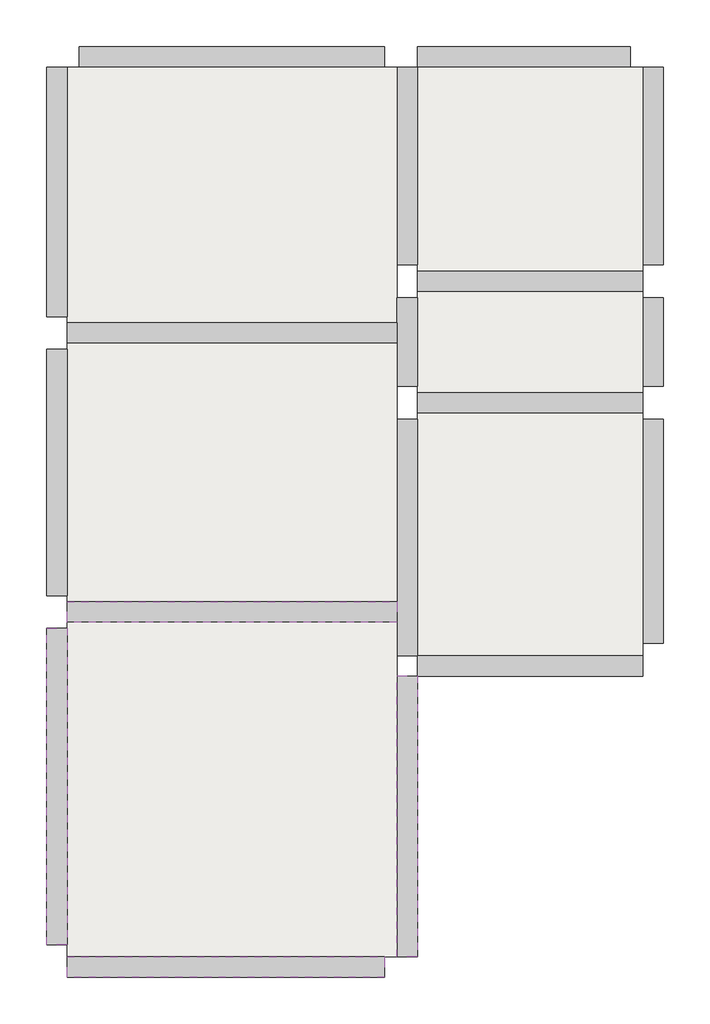
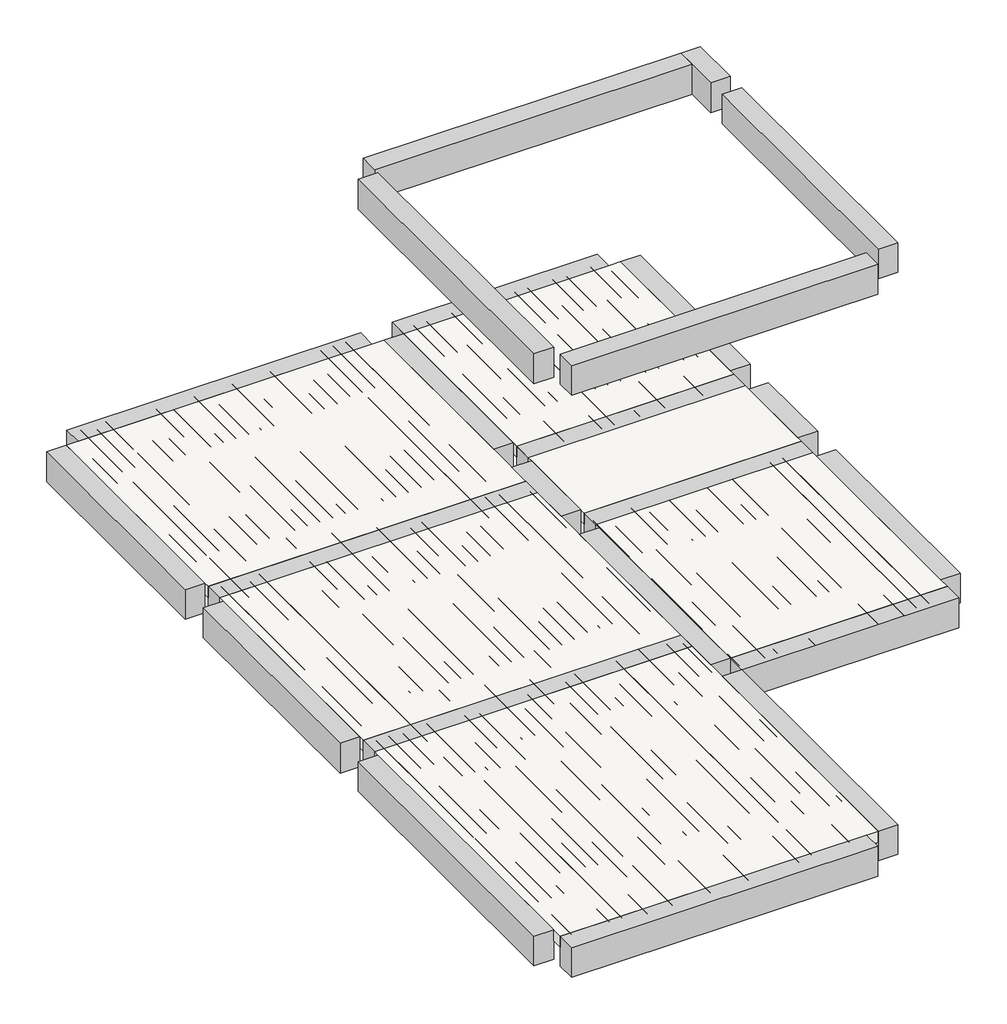
# One storey, part 1 of 2: 22 beams, 6 slabs.
"""IFC4 building model written with IfcOpenShell, lengths in millimetres."""

from ifc_helpers import new_model, si_unit, frame, origin, place, context, project, spatial, polyline, outline, extrude, faceted_brep, element, save

model = new_model("IFC4")

# Units and contexts
model_context = context("Model", 3, world=origin())
ifc_project = project(units=[si_unit("LENGTHUNIT", "METRE", prefix="MILLI")], contexts=[model_context])

# Site, building, storey
site = spatial("IfcSite", under=ifc_project)
building = spatial("IfcBuilding", under=site)
storey = spatial("IfcBuildingStorey", under=building, Elevation=0.0)

# Beams
placement = place(None, origin())
element("IfcBeam", 1, ObjectType="Concrete-Rectangular Beam : BEAM", at=placement, inside=storey, context=model_context, shape_type="SweptSolid", body=[
    extrude(outline(polyline([(-12336.5990423, 3901.2699494), (-12082.5990423, 3901.2699494), (-12082.5990423, -16.6800506), (-12336.5990423, -16.6800506), (-12336.5990423, 3901.2699494)])), frame((0.0, 0.0, -406.4), z_axis=(0.0, 0.0, 1.0), x_axis=(1.0, 0.0, 0.0)), (0.0, 0.0, 1.0), 406.4),
])
element("IfcBeam", 2, ObjectType="Concrete-Rectangular Beam : BEAM", at=placement, inside=storey, context=model_context, shape_type="SweptSolid", body=[
    extrude(outline(polyline([(-12336.5990423, 7355.6699494), (-12082.5990423, 7355.6699494), (-12082.5990423, 4307.6699494), (-12336.5990423, 4307.6699494), (-12336.5990423, 7355.6699494)])), frame((0.0, 0.0, -406.4), z_axis=(0.0, 0.0, 1.0), x_axis=(1.0, 0.0, 0.0)), (0.0, 0.0, 1.0), 406.4),
])
element("IfcBeam", 3, ObjectType="Concrete-Rectangular Beam : BEAM", at=placement, inside=storey, context=model_context, shape_type="Brep", body=[
    faceted_brep([(-12082.5990423, 10854.5199494, 0.0), (-12336.5990423, 10854.5199494, 0.0), (-12336.5990423, 7762.0699494, 0.0), (-12082.5990423, 7762.0699494, 0.0), (-12082.5990423, 10854.5199494, -406.4), (-12082.5990423, 10854.5199494, -152.4), (-12082.5990423, 7762.0699494, -406.4), (-12336.5990423, 10854.5199494, -406.4), (-12336.5990423, 7762.0699494, -406.4)], [[[0, 1, 2, 3]], [[4, 5, 0, 3, 6]], [[7, 4, 6, 8]], [[1, 7, 8, 2]], [[1, 0, 5, 4, 7]], [[3, 2, 8, 6]]]),
])
element("IfcBeam", 4, ObjectType="Concrete-Rectangular Beam : BEAM", at=placement, inside=storey, context=model_context, shape_type="SweptSolid", body=[
    extrude(outline(polyline([(-11930.1990423, 10854.5199494), (-11930.1990423, 11108.5199494), (-8145.5990423, 11108.5199494), (-8145.5990423, 10854.5199494), (-11930.1990423, 10854.5199494)])), frame((0.0, 0.0, -406.4), z_axis=(0.0, 0.0, 1.0), x_axis=(1.0, 0.0, 0.0)), (0.0, 0.0, 1.0), 406.4),
])
element("IfcBeam", 5, ObjectType="Concrete-Rectangular Beam : BEAM", at=placement, inside=storey, context=model_context, shape_type="Brep", body=[
    faceted_brep([(-7739.1990423, 11108.5199494, 0.0), (-7739.1990423, 10854.5199494, 0.0), (-5097.5990423, 10854.5199494, 0.0), (-5097.5990423, 11108.5199494, 0.0), (-7739.1990423, 10854.5199494, -152.4), (-7739.1990423, 10854.5199494, -406.4), (-5097.5990423, 10854.5199494, -406.4), (-7739.1990423, 11108.5199494, -406.4), (-5097.5990423, 11108.5199494, -406.4)], [[[0, 1, 2, 3]], [[1, 4, 5, 6, 2]], [[5, 7, 8, 6]], [[7, 0, 3, 8]], [[1, 0, 7, 5, 4]], [[3, 2, 6, 8]]]),
])
element("IfcBeam", 6, ObjectType="Concrete-Rectangular Beam : BEAM", at=placement, inside=storey, context=model_context, shape_type="Brep", body=[
    faceted_brep([(-4945.1990423, 8403.4199494, 0.0), (-4691.1990423, 8403.4199494, 0.0), (-4691.1990423, 10854.5199494, 0.0), (-4945.1990423, 10854.5199494, 0.0), (-4691.1990423, 8403.4199494, -406.4), (-4691.1990423, 10854.5199494, -406.4), (-4945.1990423, 8403.4199494, -406.4), (-4945.1990423, 10854.5199494, -406.4), (-4945.1990423, 10854.5199494, -152.4)], [[[0, 1, 2, 3]], [[1, 4, 5, 2]], [[4, 6, 7, 5]], [[6, 0, 3, 8, 7]], [[1, 0, 6, 4]], [[2, 5, 7, 8, 3]]]),
])
element("IfcBeam", 7, ObjectType="Concrete-Rectangular Beam : BEAM", at=placement, inside=storey, context=model_context, shape_type="SweptSolid", body=[
    extrude(outline(polyline([(-4945.1990423, 7997.0199494), (-4691.1990423, 7997.0199494), (-4691.1990423, 6898.4699494), (-4945.1990423, 6898.4699494), (-4945.1990423, 7997.0199494)])), frame((0.0, 0.0, -406.4), z_axis=(0.0, 0.0, 1.0), x_axis=(1.0, 0.0, 0.0)), (0.0, 0.0, 1.0), 406.4),
])
element("IfcBeam", 8, ObjectType="Concrete-Rectangular Beam : BEAM", at=placement, inside=storey, context=model_context, shape_type="SweptSolid", body=[
    extrude(outline(polyline([(-4691.1990423, 3717.1199494), (-4945.1990423, 3717.1199494), (-4945.1990423, 6492.0699494), (-4691.1990423, 6492.0699494), (-4691.1990423, 3717.1199494)])), frame((0.0, 0.0, -406.4), z_axis=(0.0, 0.0, 1.0), x_axis=(1.0, 0.0, 0.0)), (0.0, 0.0, 1.0), 406.4),
])
element("IfcBeam", 9, ObjectType="Concrete-Rectangular Beam : BEAM", at=placement, inside=storey, context=model_context, shape_type="Brep", body=[
    faceted_brep([(-7739.1990423, 3564.7199494, 0.0), (-7739.1990423, 3310.7199494, 0.0), (-4945.1990423, 3310.7199494, 0.0), (-4945.1990423, 3564.7199494, 0.0), (-7739.1990423, 3564.7199494, -406.4), (-7739.1990423, 3564.7199494, -152.4), (-4945.1990423, 3564.7199494, -152.4), (-4945.1990423, 3564.7199494, -406.4), (-7739.1990423, 3310.7199494, -406.4), (-4945.1990423, 3310.7199494, -406.4)], [[[0, 1, 2, 3]], [[4, 5, 0, 3, 6, 7]], [[8, 4, 7, 9]], [[1, 8, 9, 2]], [[1, 0, 5, 4, 8]], [[2, 9, 7, 6, 3]]]),
])
element("IfcBeam", 10, ObjectType="Concrete-Rectangular Beam : BEAM", at=placement, inside=storey, context=model_context, shape_type="Brep", body=[
    faceted_brep([(-7993.1990423, 3564.7199494, 0.0), (-7739.1990423, 3564.7199494, 0.0), (-7739.1990423, 6492.0699494, 0.0), (-7993.1990423, 6492.0699494, 0.0), (-7993.1990423, 4231.4699494, 0.0), (-7993.1990423, 3977.4699494, 0.0), (-7993.1990423, 3564.7199494, -406.4), (-7993.1990423, 6492.0699494, -406.4), (-7993.1990423, 4231.4699494, -406.4), (-7993.1990423, 3977.4699494, -406.4), (-7739.1990423, 3564.7199494, -406.4), (-7739.1990423, 6492.0699494, -406.4), (-7739.1990423, 3564.7199494, -152.4)], [[[0, 1, 2, 3, 4, 5]], [[6, 0, 5, 4, 3, 7, 8, 9]], [[10, 6, 9, 8, 7, 11]], [[1, 12, 10, 11, 2]], [[10, 12, 1, 0, 6]], [[3, 2, 11, 7]]]),
])
element("IfcBeam", 11, ObjectType="Concrete-Rectangular Beam : BEAM", at=placement, inside=storey, context=model_context, shape_type="Brep", body=[
    faceted_brep([(-7993.1990423, 6898.4699494, 0.0), (-7739.1990423, 6898.4699494, 0.0), (-7739.1990423, 7997.0199494, 0.0), (-7993.1990423, 7997.0199494, 0.0), (-7993.1990423, 7685.8699494, 0.0), (-7993.1990423, 7431.8699494, 0.0), (-7739.1990423, 6898.4699494, -406.4), (-7739.1990423, 7997.0199494, -406.4), (-7993.1990423, 6898.4699494, -406.4), (-7993.1990423, 7431.8699494, -406.4), (-7993.1990423, 7685.8699494, -406.4), (-7993.1990423, 7997.0199494, -406.4)], [[[0, 1, 2, 3, 4, 5]], [[1, 6, 7, 2]], [[6, 8, 9, 10, 11, 7]], [[8, 0, 5, 4, 3, 11, 10, 9]], [[1, 0, 8, 6]], [[3, 2, 7, 11]]]),
])
element("IfcBeam", 12, ObjectType="Concrete-Rectangular Beam : BEAM", at=placement, inside=storey, context=model_context, shape_type="Brep", body=[
    faceted_brep([(-7739.1990423, 10854.5199494, 0.0), (-7993.1990423, 10854.5199494, 0.0), (-7993.1990423, 8403.4199494, 0.0), (-7739.1990423, 8403.4199494, 0.0), (-7739.1990423, 10854.5199494, -406.4), (-7739.1990423, 10854.5199494, -152.4), (-7739.1990423, 8403.4199494, -406.4), (-7993.1990423, 10854.5199494, -406.4), (-7993.1990423, 8403.4199494, -406.4), (-7993.1990423, 10854.5199494, -152.4)], [[[0, 1, 2, 3]], [[4, 5, 0, 3, 6]], [[7, 4, 6, 8]], [[1, 9, 7, 8, 2]], [[7, 9, 1, 0, 5, 4]], [[3, 2, 8, 6]]]),
])
element("IfcBeam", 13, ObjectType="Concrete-Rectangular Beam : BEAM", at=placement, inside=storey, context=model_context, shape_type="Brep", body=[
    faceted_brep([(-7739.1990423, 3310.7199494, 0.0), (-7993.1990423, 3310.7199494, 0.0), (-7993.1990423, -169.0800506, 0.0), (-7739.1990423, -169.0800506, 0.0), (-7993.1990423, 3310.7199494, -406.4), (-7993.1990423, -169.0800506, -406.4), (-7993.1990423, -169.0800506, -152.4), (-7739.1990423, 3310.7199494, -406.4), (-7739.1990423, -169.0800506, -406.4)], [[[0, 1, 2, 3]], [[1, 4, 5, 6, 2]], [[4, 7, 8, 5]], [[7, 0, 3, 8]], [[0, 7, 4, 1]], [[3, 2, 6, 5, 8]]]),
])
element("IfcBeam", 14, ObjectType="Concrete-Rectangular Beam : BEAM", at=placement, inside=storey, context=model_context, shape_type="Brep", body=[
    faceted_brep([(-12082.5990423, -169.0800506, 0.0), (-12082.5990423, -423.0800506, 0.0), (-8145.5990423, -423.0800506, 0.0), (-8145.5990423, -169.0800506, 0.0), (-12082.5990423, -169.0800506, -406.4), (-12082.5990423, -169.0800506, -152.4), (-8145.5990423, -169.0800506, -406.4), (-12082.5990423, -423.0800506, -406.4), (-8145.5990423, -423.0800506, -406.4)], [[[0, 1, 2, 3]], [[4, 5, 0, 3, 6]], [[7, 4, 6, 8]], [[1, 7, 8, 2]], [[0, 5, 4, 7, 1]], [[3, 2, 8, 6]]]),
])
element("IfcBeam", 15, ObjectType="Concrete-Rectangular Beam : BEAM", at=placement, inside=storey, context=model_context, shape_type="Brep", body=[
    faceted_brep([(-12082.5990423, 7685.8699494, 0.0), (-12082.5990423, 7431.8699494, 0.0), (-7993.1990423, 7431.8699494, 0.0), (-7993.1990423, 7685.8699494, 0.0), (-12082.5990423, 7431.8699494, -152.4), (-12082.5990423, 7431.8699494, -406.4), (-7993.1990423, 7431.8699494, -406.4), (-7993.1990423, 7431.8699494, -152.4), (-12082.5990423, 7685.8699494, -406.4), (-7993.1990423, 7685.8699494, -406.4), (-12082.5990423, 7685.8699494, -152.4), (-7993.1990423, 7685.8699494, -152.4)], [[[0, 1, 2, 3]], [[1, 4, 5, 6, 7, 2]], [[5, 8, 9, 6]], [[8, 10, 0, 3, 11, 9]], [[5, 4, 1, 0, 10, 8]], [[3, 2, 7, 6, 9, 11]]]),
])
element("IfcBeam", 16, ObjectType="Concrete-Rectangular Beam : BEAM", at=placement, inside=storey, context=model_context, shape_type="Brep", body=[
    faceted_brep([(-4945.1990423, 8073.2199494, 0.0), (-4945.1990423, 8327.2199494, 0.0), (-7739.1990423, 8327.2199494, 0.0), (-7739.1990423, 8073.2199494, 0.0), (-4945.1990423, 8073.2199494, -406.4), (-4945.1990423, 8073.2199494, -152.4), (-7739.1990423, 8073.2199494, -152.4), (-7739.1990423, 8073.2199494, -406.4), (-4945.1990423, 8327.2199494, -406.4), (-7739.1990423, 8327.2199494, -406.4), (-4945.1990423, 8327.2199494, -152.4), (-7739.1990423, 8327.2199494, -152.4)], [[[0, 1, 2, 3]], [[4, 5, 0, 3, 6, 7]], [[8, 4, 7, 9]], [[1, 10, 8, 9, 11, 2]], [[8, 10, 1, 0, 5, 4]], [[2, 11, 9, 7, 6, 3]]]),
])
element("IfcBeam", 17, ObjectType="Concrete-Rectangular Beam : BEAM", at=placement, inside=storey, context=model_context, shape_type="Brep", body=[
    faceted_brep([(-7739.1990423, 6822.2699494, 0.0), (-7739.1990423, 6568.2699494, 0.0), (-4945.1990423, 6568.2699494, 0.0), (-4945.1990423, 6822.2699494, 0.0), (-7739.1990423, 6568.2699494, -152.4), (-7739.1990423, 6568.2699494, -406.4), (-4945.1990423, 6568.2699494, -406.4), (-4945.1990423, 6568.2699494, -152.4), (-7739.1990423, 6822.2699494, -406.4), (-4945.1990423, 6822.2699494, -406.4), (-7739.1990423, 6822.2699494, -152.4), (-4945.1990423, 6822.2699494, -152.4)], [[[0, 1, 2, 3]], [[1, 4, 5, 6, 7, 2]], [[5, 8, 9, 6]], [[8, 10, 0, 3, 11, 9]], [[5, 4, 1, 0, 10, 8]], [[2, 7, 6, 9, 11, 3]]]),
])
element("IfcBeam", 18, ObjectType="Concrete-Rectangular Beam : BEAM", at=placement, inside=storey, context=model_context, shape_type="Brep", body=[
    faceted_brep([(-12082.5990423, 4231.4699494, 0.0), (-12082.5990423, 3977.4699494, 0.0), (-7993.1990423, 3977.4699494, 0.0), (-7993.1990423, 4231.4699494, 0.0), (-12082.5990423, 3977.4699494, -152.4), (-12082.5990423, 3977.4699494, -406.4), (-7993.1990423, 3977.4699494, -406.4), (-7993.1990423, 3977.4699494, -152.4), (-12082.5990423, 4231.4699494, -406.4), (-7993.1990423, 4231.4699494, -406.4), (-12082.5990423, 4231.4699494, -152.4), (-7993.1990423, 4231.4699494, -152.4)], [[[0, 1, 2, 3]], [[1, 4, 5, 6, 7, 2]], [[5, 8, 9, 6]], [[8, 10, 0, 3, 11, 9]], [[5, 4, 1, 0, 10, 8]], [[3, 2, 7, 6, 9, 11]]]),
])
element("IfcBeam", 19, ObjectType="Concrete-Rectangular Beam : BEAM", at=placement, inside=storey, context=model_context, shape_type="SweptSolid", body=[
    extrude(outline(polyline([(-12336.5990423, 3901.2699494), (-12082.5990423, 3901.2699494), (-12082.5990423, -16.6800506), (-12336.5990423, -16.6800506), (-12336.5990423, 3901.2699494)])), frame((0.0, 0.0, 7518.4), z_axis=(0.0, 0.0, 1.0), x_axis=(1.0, 0.0, 0.0)), (0.0, 0.0, 1.0), 406.4),
])
element("IfcBeam", 20, ObjectType="Concrete-Rectangular Beam : BEAM", at=placement, inside=storey, context=model_context, shape_type="Brep", body=[
    faceted_brep([(-7993.1990423, 3564.7199494, 7924.8), (-7739.1990423, 3564.7199494, 7924.8), (-7739.1990423, 4231.4699494, 7924.8), (-7993.1990423, 4231.4699494, 7924.8), (-7993.1990423, 3977.4699494, 7924.8), (-7993.1990423, 3564.7199494, 7518.4), (-7993.1990423, 4231.4699494, 7518.4), (-7993.1990423, 3977.4699494, 7518.4), (-7739.1990423, 3564.7199494, 7518.4), (-7739.1990423, 4231.4699494, 7518.4)], [[[0, 1, 2, 3, 4]], [[5, 0, 4, 3, 6, 7]], [[8, 5, 7, 6, 9]], [[1, 8, 9, 2]], [[1, 0, 5, 8]], [[3, 2, 9, 6]]]),
    faceted_brep([(-7993.1990423, 3310.7199494, 7924.8), (-7739.1990423, 3310.7199494, 7924.8), (-7739.1990423, 3310.7199494, 7518.4), (-7993.1990423, 3310.7199494, 7518.4), (-7739.1990423, -169.0800506, 7924.8), (-7993.1990423, -169.0800506, 7924.8), (-7993.1990423, -169.0800506, 7518.4), (-7739.1990423, -169.0800506, 7518.4)], [[[0, 1, 2, 3]], [[4, 5, 6, 7]], [[1, 0, 5, 4]], [[0, 3, 6, 5]], [[3, 2, 7, 6]], [[2, 1, 4, 7]]]),
])
element("IfcBeam", 21, ObjectType="Concrete-Rectangular Beam : BEAM", at=placement, inside=storey, context=model_context, shape_type="SweptSolid", body=[
    extrude(outline(polyline([(-12082.5990423, -423.0800506), (-12082.5990423, -169.0800506), (-8145.5990423, -169.0800506), (-8145.5990423, -423.0800506), (-12082.5990423, -423.0800506)])), frame((0.0, 0.0, 7518.4), z_axis=(0.0, 0.0, 1.0), x_axis=(1.0, 0.0, 0.0)), (0.0, 0.0, 1.0), 406.4),
])
element("IfcBeam", 22, ObjectType="Concrete-Rectangular Beam : BEAM", at=placement, inside=storey, context=model_context, shape_type="SweptSolid", body=[
    extrude(outline(polyline([(-12082.5990423, 3977.4699494), (-12082.5990423, 4231.4699494), (-7993.1990423, 4231.4699494), (-7993.1990423, 3977.4699494), (-12082.5990423, 3977.4699494)])), frame((0.0, 0.0, 7518.4), z_axis=(0.0, 0.0, 1.0), x_axis=(1.0, 0.0, 0.0)), (0.0, 0.0, 1.0), 406.4),
])

# Slabs
element("IfcSlab", 23, ObjectType="6\" Foundation Slab", at=placement, inside=storey, context=model_context, shape_type="Brep", body=[
    faceted_brep([(-7993.1990423, 10854.5199494, -152.4), (-7993.1990423, 7685.8699494, -152.4), (-12082.5990423, 7685.8699494, -152.4), (-12082.5990423, 10854.5199494, -152.4), (-7993.1990423, 10854.5199494, 0.0), (-8145.5990423, 10854.5199494, 0.0), (-11930.1990423, 10854.5199494, 0.0), (-12082.5990423, 10854.5199494, 0.0), (-12082.5990423, 7762.0699494, 0.0), (-12082.5990423, 7685.8699494, 0.0), (-7993.1990423, 7685.8699494, 0.0), (-7993.1990423, 7997.0199494, 0.0), (-7993.1990423, 8403.4199494, 0.0)], [[[0, 1, 2, 3]], [[4, 5, 6, 7, 8, 9, 10, 11, 12]], [[1, 0, 4, 12, 11, 10]], [[2, 1, 10, 9]], [[3, 2, 9, 8, 7]], [[0, 3, 7, 6, 5, 4]]]),
])
element("IfcSlab", 24, ObjectType="6\" Foundation Slab", at=placement, inside=storey, context=model_context, shape_type="Brep", body=[
    faceted_brep([(-4945.1990423, 10854.5199494, -152.4), (-4945.1990423, 8327.2199494, -152.4), (-7739.1990423, 8327.2199494, -152.4), (-7739.1990423, 10854.5199494, -152.4), (-4945.1990423, 10854.5199494, 0.0), (-5097.5990423, 10854.5199494, 0.0), (-7739.1990423, 10854.5199494, 0.0), (-7739.1990423, 8403.4199494, 0.0), (-7739.1990423, 8327.2199494, 0.0), (-4945.1990423, 8327.2199494, 0.0), (-4945.1990423, 8403.4199494, 0.0)], [[[0, 1, 2, 3]], [[4, 5, 6, 7, 8, 9, 10]], [[1, 0, 4, 10, 9]], [[2, 1, 9, 8]], [[3, 2, 8, 7, 6]], [[0, 3, 6, 5, 4]]]),
])
element("IfcSlab", 25, ObjectType="6\" Foundation Slab", at=placement, inside=storey, context=model_context, shape_type="Brep", body=[
    faceted_brep([(-7993.1990423, 7431.8699494, -152.4), (-7993.1990423, 4231.4699494, -152.4), (-12082.5990423, 4231.4699494, -152.4), (-12082.5990423, 7431.8699494, -152.4), (-7993.1990423, 7431.8699494, 0.0), (-12082.5990423, 7431.8699494, 0.0), (-12082.5990423, 7355.6699494, 0.0), (-12082.5990423, 4307.6699494, 0.0), (-12082.5990423, 4231.4699494, 0.0), (-7993.1990423, 4231.4699494, 0.0), (-7993.1990423, 6492.0699494, 0.0), (-7993.1990423, 6898.4699494, 0.0)], [[[0, 1, 2, 3]], [[4, 5, 6, 7, 8, 9, 10, 11]], [[1, 0, 4, 11, 10, 9]], [[2, 1, 9, 8]], [[3, 2, 8, 7, 6, 5]], [[0, 3, 5, 4]]]),
])
element("IfcSlab", 26, ObjectType="6\" Foundation Slab", at=placement, inside=storey, context=model_context, shape_type="Brep", body=[
    faceted_brep([(-4945.1990423, 6568.2699494, -152.4), (-4945.1990423, 3564.7199494, -152.4), (-7739.1990423, 3564.7199494, -152.4), (-7739.1990423, 6568.2699494, -152.4), (-4945.1990423, 6568.2699494, 0.0), (-7739.1990423, 6568.2699494, 0.0), (-7739.1990423, 6492.0699494, 0.0), (-7739.1990423, 3564.7199494, 0.0), (-4945.1990423, 3564.7199494, 0.0), (-4945.1990423, 3717.1199494, 0.0), (-4945.1990423, 6492.0699494, 0.0)], [[[0, 1, 2, 3]], [[4, 5, 6, 7, 8, 9, 10]], [[1, 0, 4, 10, 9, 8]], [[2, 1, 8, 7]], [[3, 2, 7, 6, 5]], [[0, 3, 5, 4]]]),
])
element("IfcSlab", 27, ObjectType="6\" Foundation Slab", at=placement, inside=storey, context=model_context, shape_type="Brep", body=[
    faceted_brep([(-7993.1990423, 3977.4699494, -152.4), (-7993.1990423, -169.0800506, -152.4), (-12082.5990423, -169.0800506, -152.4), (-12082.5990423, 3977.4699494, -152.4), (-7993.1990423, 3977.4699494, 0.0), (-12082.5990423, 3977.4699494, 0.0), (-12082.5990423, 3901.2699494, 0.0), (-12082.5990423, -16.6800506, 0.0), (-12082.5990423, -169.0800506, 0.0), (-8145.5990423, -169.0800506, 0.0), (-7993.1990423, -169.0800506, 0.0), (-7993.1990423, 3310.7199494, 0.0), (-7993.1990423, 3564.7199494, 0.0)], [[[0, 1, 2, 3]], [[4, 5, 6, 7, 8, 9, 10, 11, 12]], [[1, 0, 4, 12, 11, 10]], [[2, 1, 10, 9, 8]], [[3, 2, 8, 7, 6, 5]], [[0, 3, 5, 4]]]),
])
element("IfcSlab", 28, ObjectType="6\" Foundation Slab", at=placement, inside=storey, context=model_context, shape_type="Brep", body=[
    faceted_brep([(-4945.1990423, 8073.2199494, -152.4), (-4945.1990423, 6822.2699494, -152.4), (-7739.1990423, 6822.2699494, -152.4), (-7739.1990423, 8073.2199494, -152.4), (-4945.1990423, 8073.2199494, 0.0), (-7739.1990423, 8073.2199494, 0.0), (-7739.1990423, 7997.0199494, 0.0), (-7739.1990423, 6898.4699494, 0.0), (-7739.1990423, 6822.2699494, 0.0), (-4945.1990423, 6822.2699494, 0.0), (-4945.1990423, 6898.4699494, 0.0), (-4945.1990423, 7997.0199494, 0.0)], [[[0, 1, 2, 3]], [[4, 5, 6, 7, 8, 9, 10, 11]], [[1, 0, 4, 11, 10, 9]], [[2, 1, 9, 8]], [[3, 2, 8, 7, 6, 5]], [[0, 3, 5, 4]]]),
])

save(model, "model.ifc")

# Revit data of these elements
# Type "Concrete-Rectangular Beam : BEAM"
#   Assembly Code = "B10"
#   Length [instance default] = 1524 mm
#   b = 254 mm
#   h = 406.4 mm
#   Structural Material [instance default] = Concrete, Cast-in-Place gray
# Type "6\" Foundation Slab"
#   Layers, outside or top first: 152.4 mm "Concrete, Cast-in-Place gray" (function 1)
# Elements 1, 2, 3, 4, 5, 6, 7, 8, 9, 10, 11, 12, 13, 14, 15, 16, 17, 18, 19, 20, 21, 22 (IfcBeam, "Concrete-Rectangular Beam : BEAM")
#   Structural Material = Concrete, Cast-in-Place gray
#   Phase Created = New Construction
#   Materials on its faces: "Concrete, Cast-in-Place gray"
# Elements 23, 24, 25, 26, 27, 28 (IfcSlab, "6\" Foundation Slab")
#   Height Offset From Level = 0 mm
#   built-in parameter 1001954 = 1
#   Phase Created = New Construction
#   Materials on its faces: "Concrete, Cast-in-Place gray"
# Materials
#   "Concrete, Cast-in-Place gray": class "Concrete", colour RGB 192 192 192, transparency 0, Description = "Cast-in-place concrete", Cost = 0
